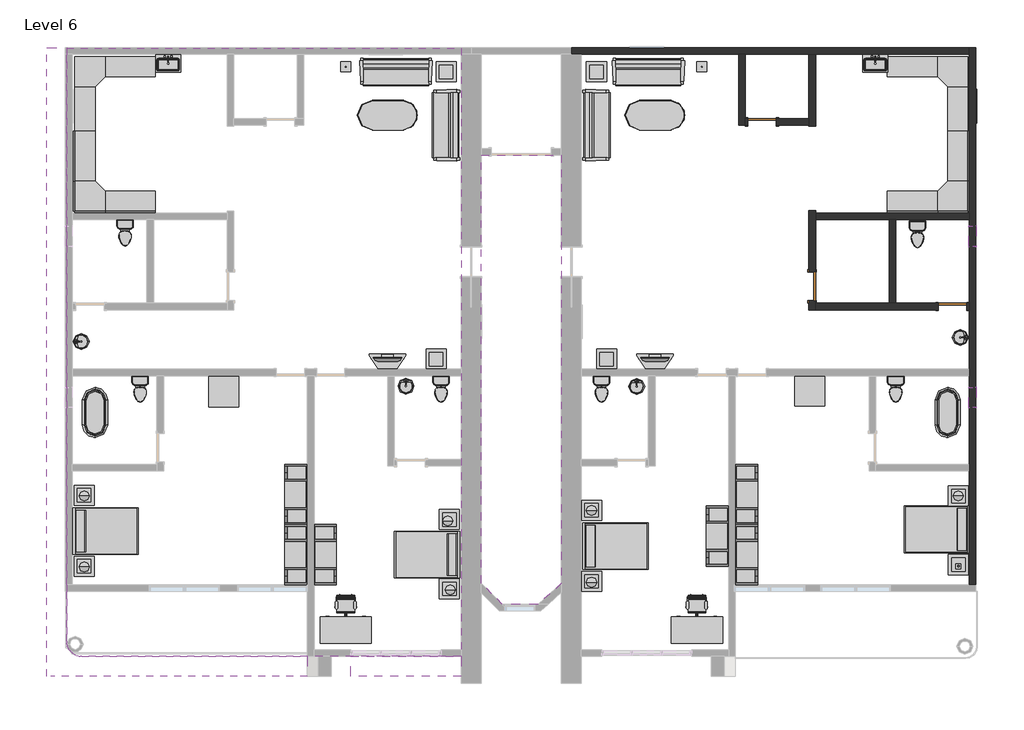
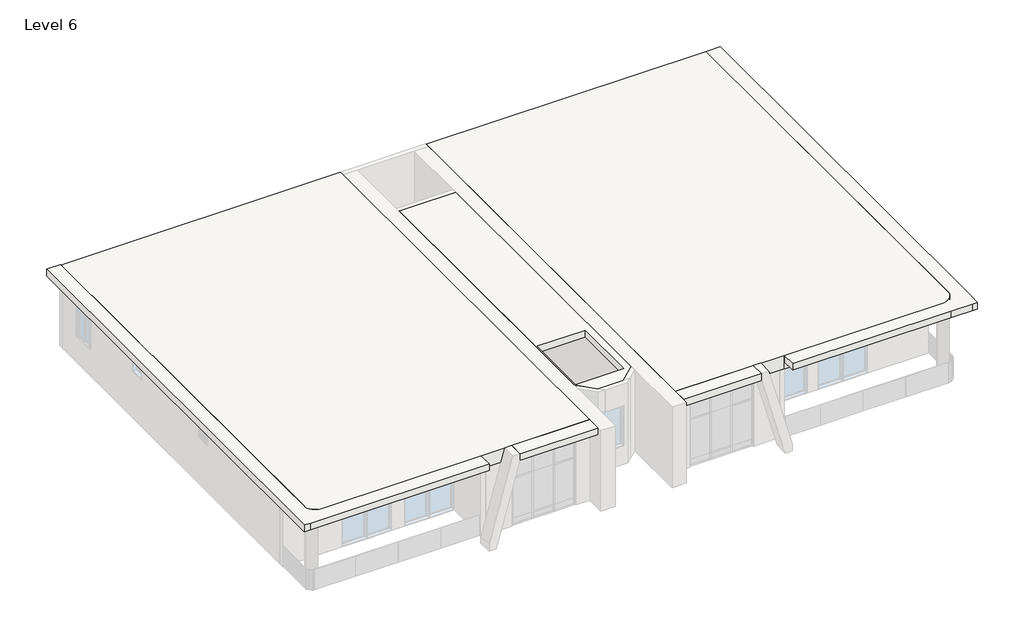
# One storey, part 3 of 3: 42 furniture elements, 14 flow terminals, 10 light fixtures, 9 walls, 4 slabs, 3 doors, 3 windows.
# Revit data of these elements (continued)
# Elements 26, 27 (IfcFurniture, "Desk : 60\" x 30\"")
#   Phase Created = New Construction
#   Materials on its faces: "Steel, Chrome Plated", "Laminate, Ivory, Matte", "Cherry"
# Elements 28, 29, 30, 31, 32, 33 (IfcFurniture, "Entertainment Center : 72\" x 72\" x 24\"")
#   Phase Created = New Construction
#   Materials on its faces: "Steel, Chrome Plated", "Glass - Clear, Grey"
# Elements 34, 35, 36, 37 (IfcFurniture, "Sofa-Pensi : 84\"")
#   Phase Created = New Construction
#   Materials on its faces: "Cherry", "Linen, Beige", "Steel, Chrome Plated"
# Elements 38, 39 (IfcFurniture, "TV - Flat Screen : 32\"")
#   Stand = yes
#   Phase Created = New Construction
#   Materials on its faces: "TV - Black", "TV - Glass", "TV - Screen"
# Elements 40, 41 (IfcFurniture, "TV Stand : TV Stand")
#   Phase Created = New Construction
#   Materials on its faces: "Melamine - Gray", "Glass - Shelves"
# Elements 42, 43, 44, 45, 46, 47, 48, 49, 50, 51, 52, 53 (IfcFurniture, "Table-Coffee : 24\" x 24\" x 24\"")
#   Phase Created = New Construction
#   Materials on its faces: "Glass - Clear, Grey"
# Elements 54, 55 (IfcFurniture, "Table-Dining Oval : 36\" x 72\"")
#   Phase Created = New Construction
#   Materials on its faces: "Steel, Chrome Plated", "Glass - Clear, Grey"
# Elements 56, 57 (IfcFurniture, "Table-Rectangular : 36\" x 36\"")
#   Phase Created = New Construction
#   Materials on its faces: "Birch"
# Elements 58, 59 (IfcFurniture, "Work Station Cubicle : 96\" x 96\"")
#   Phase Created = New Construction
#   Materials on its faces: "Textile - Light Gray", "Laminate, Ivory, Matte"
# Element 60 (IfcLightFixture, "100W - 120V")
#   Mark = "74"
#   Phase Created = New Construction
#   Materials on its faces: "Steel, Chrome Plated", "Glass, Frosted"
# Element 61 (IfcLightFixture, "100W - 120V")
#   Mark = "75"
#   Phase Created = New Construction
#   Materials on its faces: "Steel, Chrome Plated", "Glass, Frosted"
# Element 62 (IfcLightFixture, "Table Lamp - Hemispheric : 60W - 120V")
#   Mark = "76"
#   Phase Created = New Construction
#   Materials on its faces: "Steel, Chrome Plated", "Glass, Frosted", "Birch"
# Element 63 (IfcLightFixture, "Table Lamp - Hemispheric : 60W - 120V")
#   Mark = "77"
#   Phase Created = New Construction
#   Materials on its faces: "Steel, Chrome Plated", "Glass, Frosted", "Birch"
# Element 64 (IfcLightFixture, "Table Lamp - Hemispheric : 60W - 120V")
#   Mark = "78"
#   Phase Created = New Construction
#   Materials on its faces: "Steel, Chrome Plated", "Glass, Frosted", "Birch"
# Element 65 (IfcLightFixture, "Table Lamp - Hemispheric : 60W - 120V")
#   Mark = "79"
#   Phase Created = New Construction
#   Materials on its faces: "Steel, Chrome Plated", "Glass, Frosted", "Birch"
# Element 66 (IfcLightFixture, "Table Lamp - Hemispheric : 60W - 120V")
#   Mark = "80"
#   Phase Created = New Construction
#   Materials on its faces: "Steel, Chrome Plated", "Glass, Frosted", "Birch"
# Element 67 (IfcLightFixture, "Table Lamp - Hemispheric : 60W - 120V")
#   Mark = "81"
#   Phase Created = New Construction
#   Materials on its faces: "Steel, Chrome Plated", "Glass, Frosted", "Birch"
# Element 68 (IfcLightFixture, "Table Lamp - Hemispheric : 60W - 120V")
#   Mark = "82"
#   Phase Created = New Construction
#   Materials on its faces: "Steel, Chrome Plated", "Glass, Frosted", "Birch"
# Element 69 (IfcLightFixture, "Table Lamp - Hemispheric : 60W - 120V")
#   Mark = "83"
#   Phase Created = New Construction
#   Materials on its faces: "Steel, Chrome Plated", "Glass, Frosted", "Birch"
# Element 70 (IfcSlab, "Generic - 12\" cream")
#   Height Offset From Level = 12' - 0"
#   Phase Created = New Construction
#   Materials on its faces: "Parking Stripe"
# Element 71 (IfcSlab, "Generic - 12\" white")
#   built-in parameter 1001955 = 3.14159 (stored number, unit not read)
#   Height Offset From Level = 12' - 0"
#   Phase Created = New Construction
#   Materials on its faces: "Door - Frame"
# Elements 72, 73 (IfcSlab, "Generic - 12\" white")
#   Height Offset From Level = 12' - 0"
#   Phase Created = New Construction
#   Materials on its faces: "Door - Frame"
# Elements 74, 75, 76, 77, 78, 79, 80, 81 (IfcWall, "Generic - 8\" cream")
#   Top Offset = 0' - 0"
#   Base Offset = 0' - 0"
#   Unconnected Height = 10' - 0"
#   wall height = 10' - 0"
#   Phase Created = New Construction
#   Base Constraint = Level 6
#   Materials on its faces: "Parking Stripe"
# Element 82 (IfcWall, "Generic - 8\" white")
#   Top Offset = 0' - 0"
#   Base Offset = 0' - 0"
#   Unconnected Height = 10' - 0"
#   wall height = 10' - 0"
#   Phase Created = New Construction
#   Base Constraint = Level 6
#   Materials on its faces: "Door - Frame", "Parking Stripe"
# Element 83 (IfcWindow, "Louvers with Trim : 24\" x 24\"")
#   Mark = "148"
#   Phase Created = New Construction
#   Materials on its faces: "Glass", "Iron, Ductile"
# Element 84 (IfcWindow, "Louvers with Trim : 24\" x 24\"")
#   Mark = "149"
#   Phase Created = New Construction
#   Materials on its faces: "Glass", "Iron, Ductile"
# Element 85 (IfcWindow, "Slider with Trim : 36\" x 48\"")
#   Mark = "145"
#   Phase Created = New Construction
#   Materials on its faces: "Iron, Ductile", "Glass"
# Materials
#   "Wood - Birch - Solid Stained Light Low Gloss": class "Wood", colour RGB 210 159 95, transparency 0, Cost = 0
#   "Paint - Sienna": colour RGB 118 70 51, transparency 0, Cost = 0
#   "Steel, Polished": class "Metal", colour RGB 57 57 57, transparency 0, Description = "Polished steel", Cost = 0
#   "Porcelain, Linen": class "Ceramic", colour RGB 249 239 230, transparency 0, Description = "Porcelain, linen", Cost = 0
#   "Laminate, Linen, Matte": class "Plastic", colour RGB 249 239 230, transparency 0, Description = "Plastic Laminate - Linen, Matte", Cost = 0
#   "Porcelain, Ivory": class "Ceramic", colour RGB 247 247 239, transparency 0, Description = "Porcelain, ivory", Cost = 0
#   "Laminate, Ivory, Matte": class "Plastic", colour RGB 247 247 239, transparency 0, Description = "Plastic Laminate - Ivory, Matte", Cost = 0
#   "Birch": class "Wood", colour RGB 224 178 126, transparency 0, Description = "Betula Alleghaniensis", Cost = 0
#   "Linen, White": class "Textile", colour RGB 247 247 239, transparency 0, Description = "Linen, white", Cost = 0
#   "Plastic, Opaque Black": class "Plastic", colour RGB 0 0 0, transparency 0.7, Description = "Plastic, generic, opaque black", Cost = 0
#   "Textile - Slate Blue": class "Fabric", colour RGB 98 102 118, transparency 0
#   "Steel, Chrome Plated": class "Metal", colour RGB 17 17 17, transparency 0, Description = "Chromiuim plated steel", Cost = 0
#   "Cherry": class "Wood", colour RGB 226 177 128, transparency 0, Description = "Prunus Serotina", Cost = 0
#   "Linen, Beige": class "Textile", colour RGB 249 239 230, transparency 0, Description = "Linen, beige", Cost = 0
#   "Melamine - Gray": class "Wood", colour RGB 49 49 49, transparency 0
#   "Glass - Clear, Grey": class "Glass", colour RGB 252 255 255, transparency 0.64
#   "Textile - Light Gray": class "Fabric", colour RGB 204 204 204, transparency 0
#   "Glass, Frosted": class "Glass", colour RGB 250 244 225, transparency 0.55, Description = "physical material", Cost = 0
#   "Parking Stripe": class "Paint", colour RGB 250 250 91, transparency 0, Cost = 0
#   "Door - Frame": colour RGB 118 70 51, transparency 0, Cost = 0
#   "Iron, Ductile": class "Metal", colour RGB 0 0 0, transparency 0, Description = "Ductile cast iron", Cost = 0
#   "Glass": class "Glass", colour RGB 0 128 192, transparency 0.75, Description = "Soda Lime Glass", Cost = 0
#   "TV - Black": colour RGB 49 49 49, transparency 0
#   "TV - Glass": colour RGB 157 157 157, transparency 0.9
#   "TV - Screen": colour RGB 0 0 0, transparency 0
#   "Glass - Shelves": class "Glass", colour RGB 167 167 167, transparency 0.9
